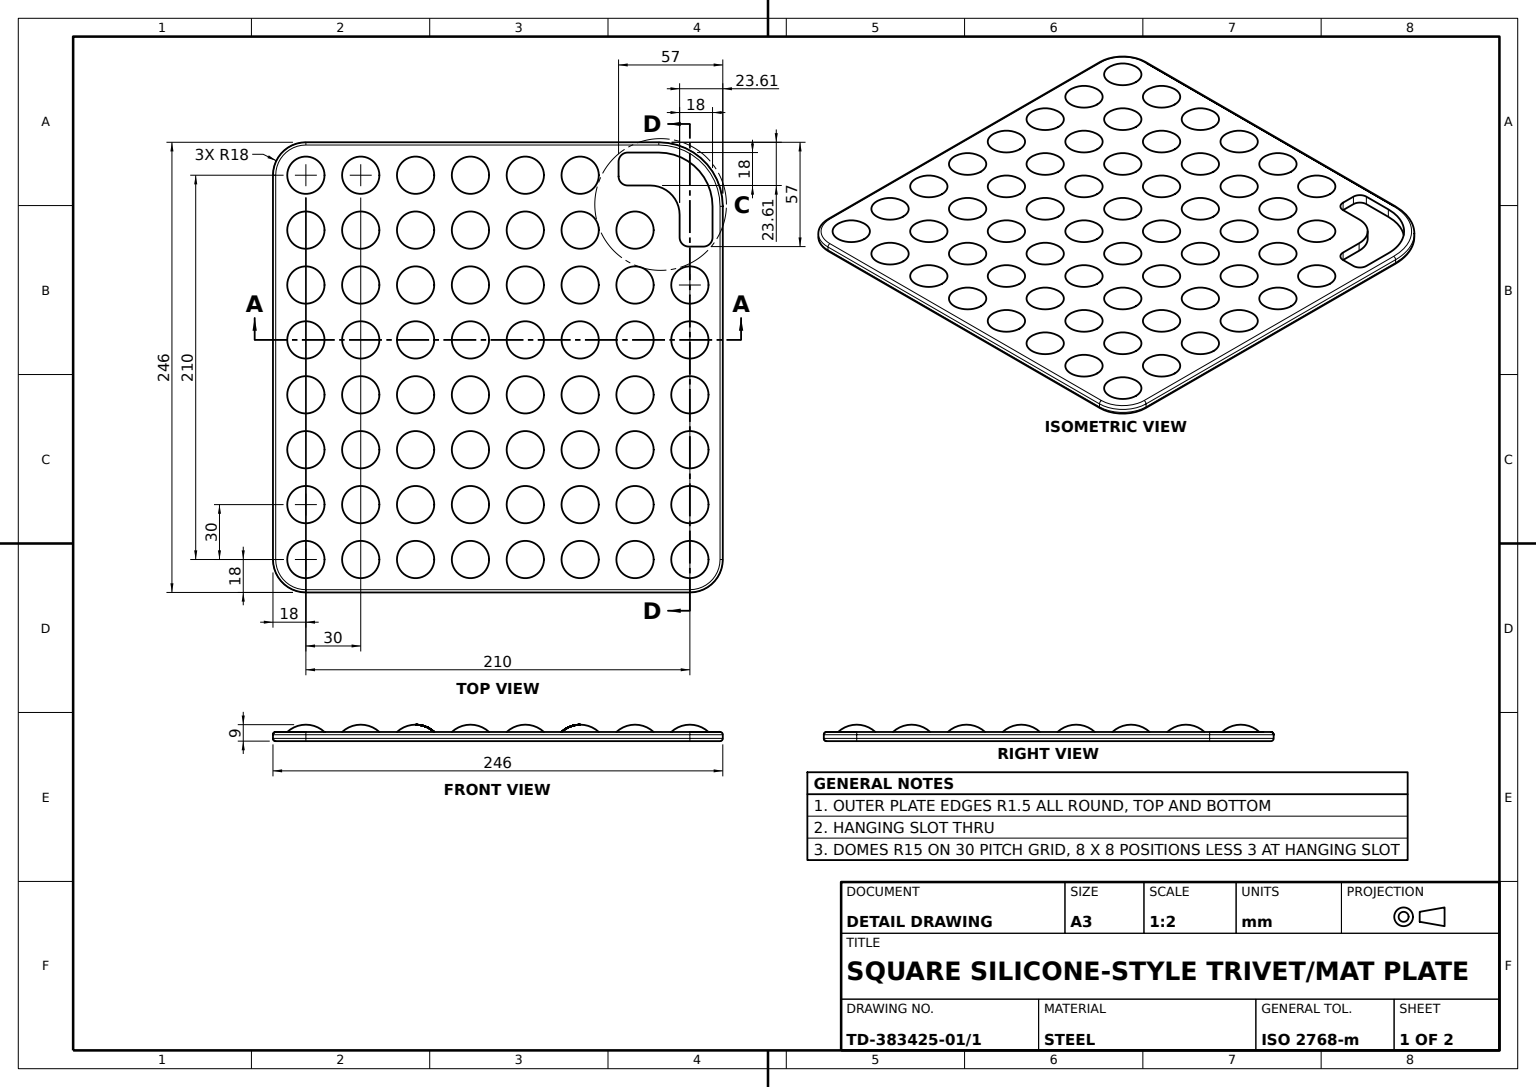
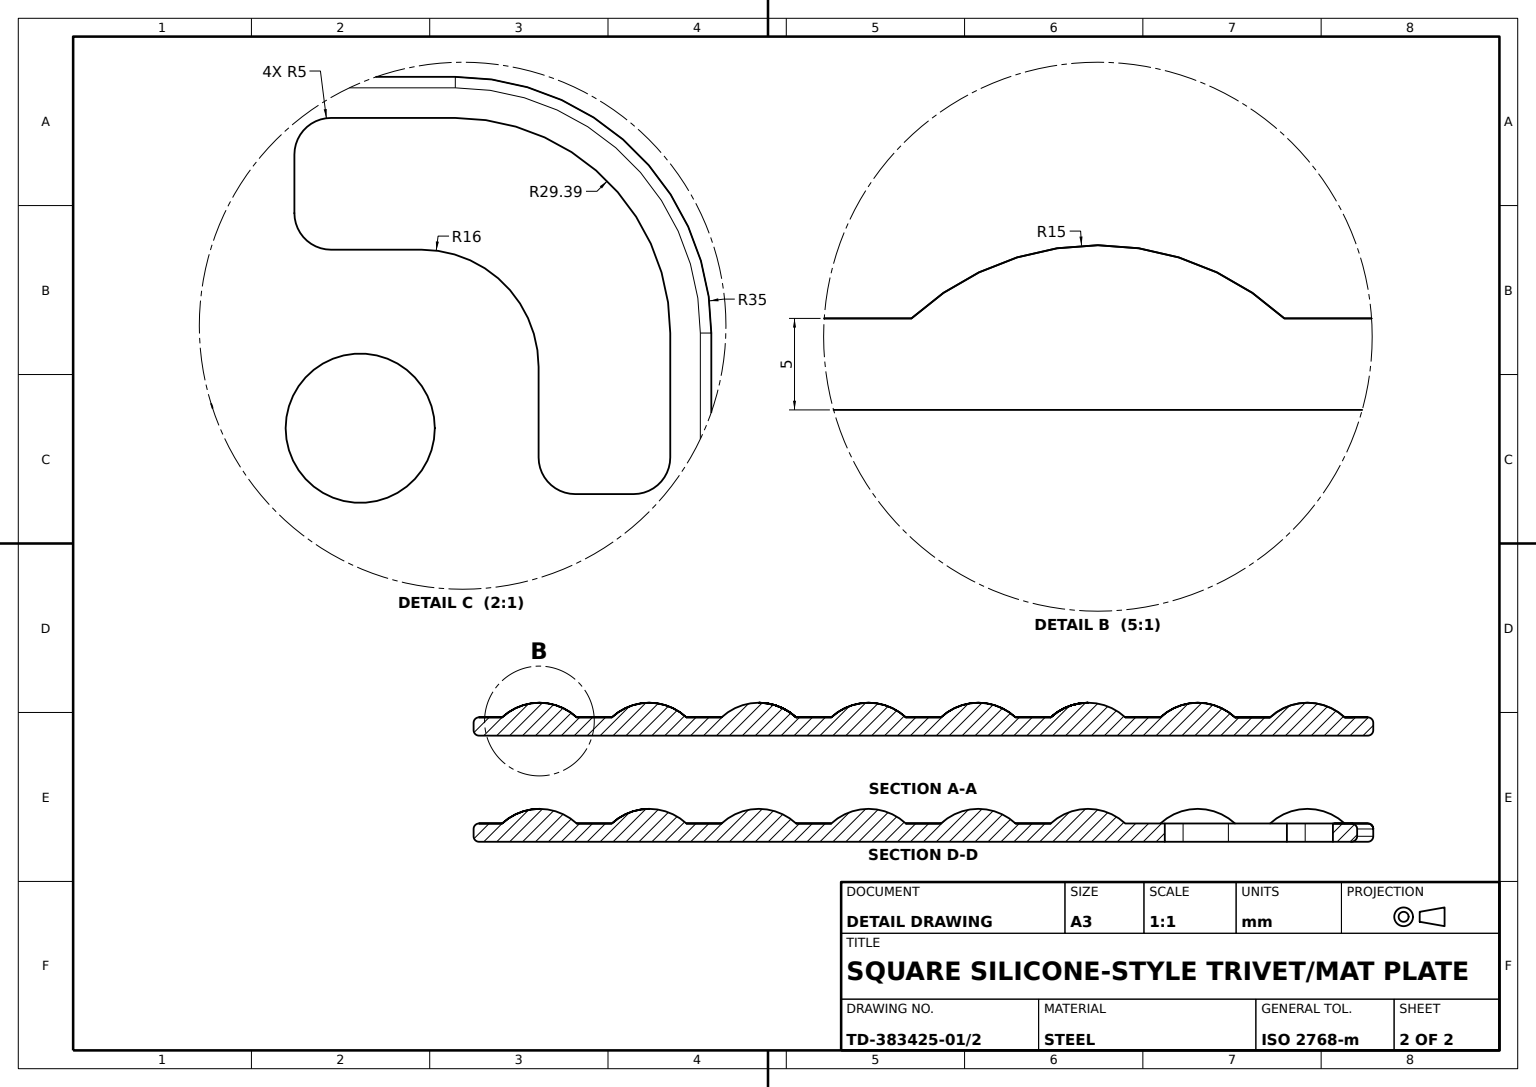
from build123d import *

# Parameters (mm, degrees)
PLATE_PROFILE_SKETCH_W                 = 246
PLATE_PROFILE_SKETCH_H                 = 246
BASE_PLATE_246X246X5_DEPTH             = 5
CORNER_FILLETS_R35_R                   = 35
HANGING_SLOT_CUT_DEPTH                 = 12.5
EDGE_FILLET_R18_R                      = 18
DOME_PATTERN_8X8_30MM_PITCH_COUNT      = 8
DOME_PATTERN_8X8_30MM_PITCH_PITCH      = 30
DOME_PATTERN_8X8_30MM_PITCH_COUNT_DIR2 = 8
DOME_PATTERN_8X8_30MM_PITCH_PITCH_DIR2 = 30
EDGE_FILLETS_R1_5_R                    = 1.5


with BuildPart() as part:
    # Plate Profile Sketch → Base Plate 246x246x5 (new body)
    with BuildSketch(Plane(origin=(0, 0, 0), x_dir=(1, 0, 0), z_dir=(0, 1, 0))):
        Rectangle(PLATE_PROFILE_SKETCH_W, PLATE_PROFILE_SKETCH_H)
    extrude(amount=BASE_PLATE_246X246X5_DEPTH)

    # Corner Fillets R35
    corner_fillets_r35_edges = [part.edges().sort_by_distance(p)[0] for p in [
        (123, 2.5, -123),
    ]]
    fillet(corner_fillets_r35_edges, radius=CORNER_FILLETS_R35_R)

    # Hanging Slot Sketch → Hanging Slot Cut (cut, symmetric)
    with BuildSketch(Plane(origin=(0, 5, 0), x_dir=(1, 0, 0), z_dir=(0, 1, 0))):
        with BuildLine():
            Line((88, 117.387520694), (71, 117.387520694))
            ThreePointArc((71, 117.387520694), (67.464466094, 115.9230546), (66, 112.387520694))
            Line((66, 112.387520694), (66, 104.387520694))
            ThreePointArc((66, 104.387520694), (67.464466094, 100.851986788), (71, 99.387520694))
            Line((71, 99.387520694), (83.387520694, 99.387520694))
            ThreePointArc((83.387520694, 99.387520694), (94.701229193, 94.701229193), (99.387520694, 83.387520694))
            Line((99.387520694, 83.387520694), (99.387520694, 71))
            ThreePointArc((99.387520694, 71), (100.851986788, 67.464466094), (104.387520694, 66))
            Line((104.387520694, 66), (112.387520694, 66))
            ThreePointArc((112.387520694, 66), (115.9230546, 67.464466094), (117.387520694, 71))
            Line((117.387520694, 71), (117.387520694, 88))
            ThreePointArc((117.387520694, 88), (108.780115165, 108.780115165), (88, 117.387520694))
        make_face()
    extrude(amount=HANGING_SLOT_CUT_DEPTH, both=True, mode=Mode.SUBTRACT)

    # Edge Fillet R18
    edge_fillet_r18_edges = [part.edges().sort_by_distance(p)[0] for p in [
        (123, 2.5, 123),
        (-123, 2.5, 123),
        (-123, 2.5, -123),
    ]]
    fillet(edge_fillet_r18_edges, radius=EDGE_FILLET_R18_R)

    # Dome Profile Sketch → Dome Boss (revolve)
    with BuildSketch(Plane.XY.offset(105), mode=Mode.PRIVATE) as dome_boss_sk:
        with BuildLine():
            Line((105, 9), (105, 5))
            Line((105, 5), (94.801960973, 5))
            ThreePointArc((94.801960973, 5), (99.522774425, 7.964240044), (105, 9))
        make_face()
    dome_boss = revolve(dome_boss_sk.sketch.rotate(Axis((105, 9, 105), (0, -1, 0)), 180), axis=Axis((105, 9, 105), (0, -1, 0)))

    # Dome Pattern 8x8 30mm Pitch: Dome Boss 8 × 8, 3 skipped
    with Locations(*[(-j * DOME_PATTERN_8X8_30MM_PITCH_PITCH_DIR2, 0, -i * DOME_PATTERN_8X8_30MM_PITCH_PITCH) for i in range(DOME_PATTERN_8X8_30MM_PITCH_COUNT) for j in range(DOME_PATTERN_8X8_30MM_PITCH_COUNT_DIR2) if (i, j) not in ((0, 0), (6, 0), (7, 0), (7, 1))]):
        add(dome_boss)

    # Edge Fillets R1.5
    edge_fillets_r1_5_edges = [part.edges().sort_by_distance(p)[0] for p in [
        (123, 5, 8.5),
        (0, 5, 123),
        (117.727922061, 5, 117.727922061),
        (-117.727922061, 5, 117.727922061),
        (-117.727922061, 5, -117.727922061),
        (-8.5, 0, -123),
        (-8.5, 5, -123),
        (112.748737342, 0, -112.748737342),
        (112.748737342, 5, -112.748737342),
        (-123, 0, 0),
        (-123, 5, 0),
        (123, 0, 8.5),
        (0, 0, 123),
        (117.727922061, 0, 117.727922061),
        (-117.727922061, 0, 117.727922061),
        (-117.727922061, 0, -117.727922061),
    ]]
    fillet(edge_fillets_r1_5_edges, radius=EDGE_FILLETS_R1_5_R)


solid = part.part
